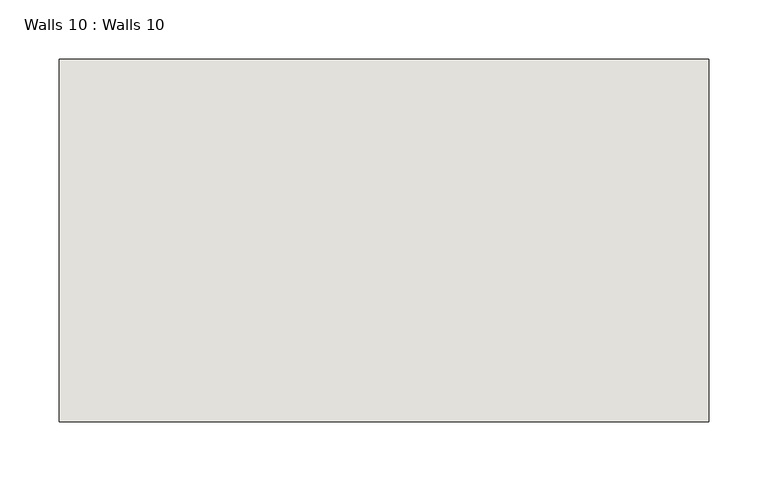
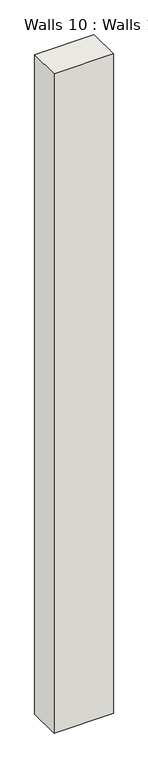
"""IFC4 building model written with IfcOpenShell, lengths in millimetres: wall geometry, Walls 10 : Walls 10."""

from ifc_helpers import new_model, si_unit, origin, origin_with_axes, place, context, project, spatial, polyline, outline, extrude, source, transform, mapped, element, save


def walls_10_walls_10_64d1ab67(model_context):
    return source(origin(), model_context, "Body", "SweptSolid", [
        extrude(outline(polyline([(-9784.4289001, -3695.7180898), (-10330.5097259, -3695.7180898), (-10330.5097259, -3390.9180898), (-9784.4289001, -3390.9180898), (-9784.4289001, -3695.7180898)])), origin_with_axes(), (0.0, 0.0, 1.0), 6400.8),
    ])


if __name__ == "__main__":
    model = new_model("IFC4")
    model_context = context("Model", 3, world=origin())
    ifc_project = project(units=[si_unit("LENGTHUNIT", "METRE", prefix="MILLI")], contexts=[model_context])
    site = spatial("IfcSite", under=ifc_project)
    building = spatial("IfcBuilding", under=site)
    placement = place(None, origin())
    walls_10_walls_10_shape = walls_10_walls_10_64d1ab67(model_context)
    element("IfcWall", 1, ObjectType="Walls 10 : Walls 10", at=placement, inside=building, context=model_context, shape_type="MappedRepresentation", body=[
        mapped(walls_10_walls_10_shape, transform((0.0, 0.0, 0.0), x_axis=(1.0, 0.0, 0.0), y_axis=(0.0, 1.0, 0.0), z_axis=(0.0, 0.0, 1.0))),
    ])
    save(model, "model.ifc")

# Revit data of these elements
# Element 1 (IfcWall, "Walls 10 : Walls 10")
#   Materials on its faces: "Default Wall"
# Materials
#   "Default Wall": colour RGB 80 80 80, transparency 0
